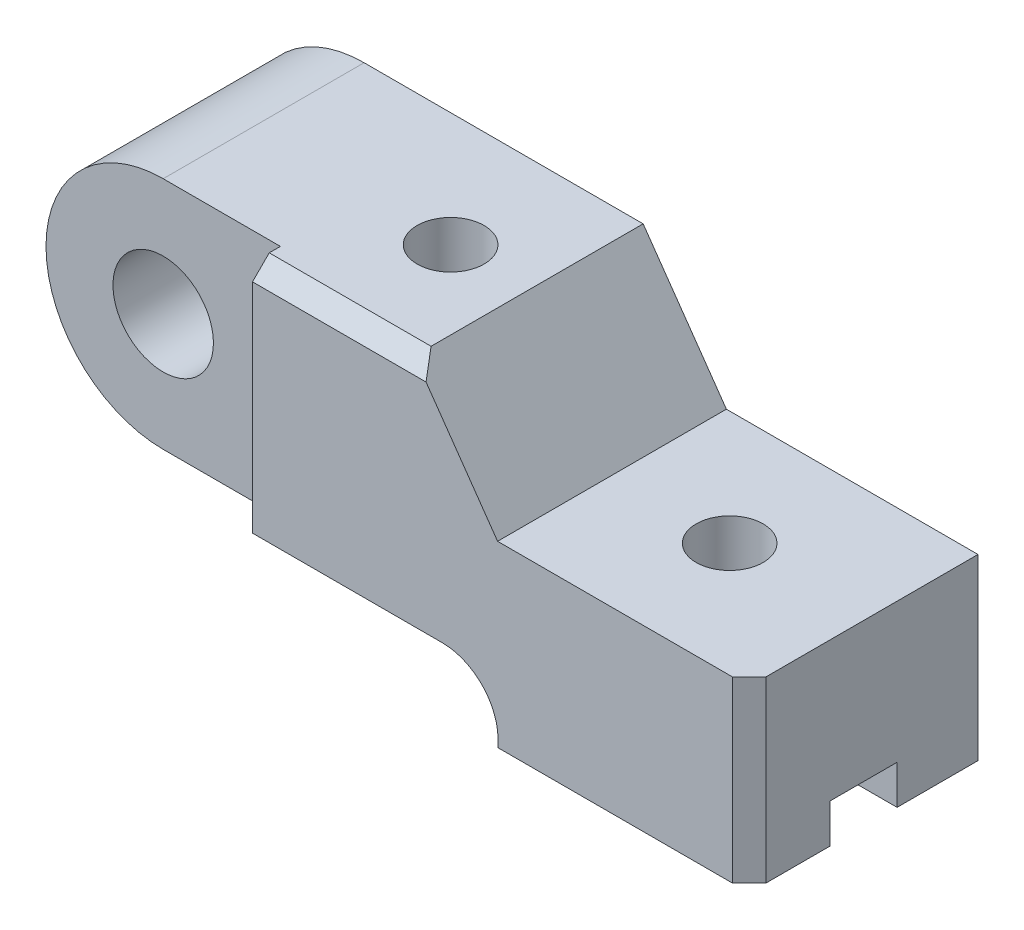
ISO-10303-21;
HEADER;
FILE_DESCRIPTION(('STEP AP214'),'2;1');
FILE_NAME('part.step','',(''),(''),'','','');
FILE_SCHEMA(('AUTOMOTIVE_DESIGN { 1 0 10303 214 1 1 1 1 }'));
ENDSEC;
DATA;
#1=APPLICATION_CONTEXT('core data for automotive mechanical design processes');
#2=APPLICATION_PROTOCOL_DEFINITION('international standard','automotive_design',2000,#1);
#3=PRODUCT_CONTEXT('',#1,'mechanical');
#4=PRODUCT('Part','Part','',(#3));
#5=PRODUCT_RELATED_PRODUCT_CATEGORY('part','',(#4));
#6=PRODUCT_DEFINITION_FORMATION('','',#4);
#7=PRODUCT_DEFINITION_CONTEXT('part definition',#1,'design');
#8=PRODUCT_DEFINITION('design','',#6,#7);
#9=PRODUCT_DEFINITION_SHAPE('','',#8);
#10=(LENGTH_UNIT() NAMED_UNIT(*) SI_UNIT(.MILLI.,.METRE.));
#11=(NAMED_UNIT(*) PLANE_ANGLE_UNIT() SI_UNIT($,.RADIAN.));
#12=(NAMED_UNIT(*) SI_UNIT($,.STERADIAN.) SOLID_ANGLE_UNIT());
#13=UNCERTAINTY_MEASURE_WITH_UNIT(LENGTH_MEASURE(1.E-05),#10,'distance_accuracy_value','');
#14=(GEOMETRIC_REPRESENTATION_CONTEXT(3) GLOBAL_UNCERTAINTY_ASSIGNED_CONTEXT((#13)) GLOBAL_UNIT_ASSIGNED_CONTEXT((#10,
#11,#12)) REPRESENTATION_CONTEXT('',''));
#15=CARTESIAN_POINT('',(0.,0.,0.));
#16=DIRECTION('',(0.,0.,1.));
#17=DIRECTION('',(1.,0.,0.));
#18=AXIS2_PLACEMENT_3D('',#15,#16,#17);
#19=CARTESIAN_POINT('',(-35.5,-25.305162605882,6.));
#20=DIRECTION('',(0.,1.,0.));
#21=DIRECTION('',(0.,0.,1.));
#22=AXIS2_PLACEMENT_3D('',#19,#20,#21);
#23=PLANE('',#22);
#24=DIRECTION('',(1.,0.,0.));
#25=VECTOR('',#24,1.);
#26=CARTESIAN_POINT('',(-35.5,-25.305162605882,6.));
#27=LINE('',#26,#25);
#28=CARTESIAN_POINT('',(86.,-25.3051626058819,6.));
#29=VERTEX_POINT('',#28);
#30=CARTESIAN_POINT('',(110.,-25.305162605882,6.));
#31=VERTEX_POINT('',#30);
#32=EDGE_CURVE('E184',#29,#31,#27,.T.);
#33=ORIENTED_EDGE('',*,*,#32,.F.);
#34=CARTESIAN_POINT('',(86.,-25.3051626058819,0.));
#35=DIRECTION('',(0.,1.,0.));
#36=DIRECTION('',(0.,0.,1.));
#37=AXIS2_PLACEMENT_3D('',#34,#35,#36);
#38=CIRCLE('',#37,6.);
#39=CARTESIAN_POINT('',(86.,-25.3051626058819,-6.00000000000001));
#40=VERTEX_POINT('',#39);
#41=EDGE_CURVE('E59',#29,#40,#38,.T.);
#42=ORIENTED_EDGE('',*,*,#41,.T.);
#43=DIRECTION('',(1.,0.,0.));
#44=VECTOR('',#43,1.);
#45=CARTESIAN_POINT('',(-35.5,-25.305162605882,-6.));
#46=LINE('',#45,#44);
#47=CARTESIAN_POINT('',(110.,-25.305162605882,-6.));
#48=VERTEX_POINT('',#47);
#49=EDGE_CURVE('E181',#40,#48,#46,.T.);
#50=ORIENTED_EDGE('',*,*,#49,.T.);
#51=DIRECTION('',(0.,0.,1.));
#52=VECTOR('',#51,1.);
#53=CARTESIAN_POINT('',(110.,-25.305162605882,6.));
#54=LINE('',#53,#52);
#55=EDGE_CURVE('E204',#48,#31,#54,.T.);
#56=ORIENTED_EDGE('',*,*,#55,.T.);
#57=EDGE_LOOP('',(#33,#42,#50,#56));
#58=FACE_BOUND('',#57,.T.);
#59=ADVANCED_FACE('F43',(#58),#23,.F.);
#60=CARTESIAN_POINT('',(65.,0.,20.5));
#61=DIRECTION('',(-1.,0.,0.));
#62=DIRECTION('',(0.,0.,1.));
#63=AXIS2_PLACEMENT_3D('',#60,#61,#62);
#64=PLANE('',#63);
#65=DIRECTION('',(0.,1.,0.));
#66=VECTOR('',#65,1.);
#67=CARTESIAN_POINT('',(65.,0.,6.));
#68=LINE('',#67,#66);
#69=CARTESIAN_POINT('',(65.,-32.305162605882,5.99999999999999));
#70=VERTEX_POINT('',#69);
#71=CARTESIAN_POINT('',(65.,-31.0000000000001,6.));
#72=VERTEX_POINT('',#71);
#73=EDGE_CURVE('E209',#70,#72,#68,.T.);
#74=ORIENTED_EDGE('',*,*,#73,.F.);
#75=DIRECTION('',(0.,0.,-1.));
#76=VECTOR('',#75,1.);
#77=CARTESIAN_POINT('',(65.,-32.305162605882,20.5));
#78=LINE('',#77,#76);
#79=CARTESIAN_POINT('',(65.,-32.305162605882,20.5));
#80=VERTEX_POINT('',#79);
#81=EDGE_CURVE('E297',#80,#70,#78,.T.);
#82=ORIENTED_EDGE('',*,*,#81,.F.);
#83=DIRECTION('',(0.,1.,0.));
#84=VECTOR('',#83,1.);
#85=CARTESIAN_POINT('',(65.,0.,20.5));
#86=LINE('',#85,#84);
#87=CARTESIAN_POINT('',(65.,-31.0000000000001,20.5));
#88=VERTEX_POINT('',#87);
#89=EDGE_CURVE('E250',#80,#88,#86,.T.);
#90=ORIENTED_EDGE('',*,*,#89,.T.);
#91=DIRECTION('',(0.,0.,-1.));
#92=VECTOR('',#91,1.);
#93=CARTESIAN_POINT('',(65.,-31.0000000000001,20.5));
#94=LINE('',#93,#92);
#95=EDGE_CURVE('E296',#88,#72,#94,.T.);
#96=ORIENTED_EDGE('',*,*,#95,.T.);
#97=EDGE_LOOP('',(#74,#82,#90,#96));
#98=FACE_BOUND('',#97,.T.);
#99=ADVANCED_FACE('F394',(#98),#64,.T.);
#100=CARTESIAN_POINT('',(0.,-32.305162605882,20.5));
#101=DIRECTION('',(0.,-1.,0.));
#102=DIRECTION('',(1.,0.,0.));
#103=AXIS2_PLACEMENT_3D('',#100,#101,#102);
#104=PLANE('',#103);
#105=DIRECTION('',(1.,0.,0.));
#106=VECTOR('',#105,1.);
#107=CARTESIAN_POINT('',(-35.5,-32.305162605882,5.99999999999999));
#108=LINE('',#107,#106);
#109=CARTESIAN_POINT('',(110.,-32.305162605882,5.99999999999999));
#110=VERTEX_POINT('',#109);
#111=EDGE_CURVE('E205',#70,#110,#108,.T.);
#112=ORIENTED_EDGE('',*,*,#111,.T.);
#113=DIRECTION('',(0.,0.,-1.));
#114=VECTOR('',#113,1.);
#115=CARTESIAN_POINT('',(110.,-32.305162605882,20.5));
#116=LINE('',#115,#114);
#117=CARTESIAN_POINT('',(110.,-32.305162605882,17.5));
#118=VERTEX_POINT('',#117);
#119=EDGE_CURVE('E295',#118,#110,#116,.T.);
#120=ORIENTED_EDGE('',*,*,#119,.F.);
#121=DIRECTION('',(0.707106781186548,0.,-0.707106781186548));
#122=VECTOR('',#121,1.);
#123=CARTESIAN_POINT('',(53.5,-32.305162605882,74.));
#124=LINE('',#123,#122);
#125=CARTESIAN_POINT('',(107.,-32.305162605882,20.5));
#126=VERTEX_POINT('',#125);
#127=EDGE_CURVE('E320',#118,#126,#124,.F.);
#128=ORIENTED_EDGE('',*,*,#127,.T.);
#129=DIRECTION('',(-1.,0.,0.));
#130=VECTOR('',#129,1.);
#131=CARTESIAN_POINT('',(0.,-32.305162605882,20.5));
#132=LINE('',#131,#130);
#133=EDGE_CURVE('E247',#126,#80,#132,.T.);
#134=ORIENTED_EDGE('',*,*,#133,.T.);
#135=ORIENTED_EDGE('',*,*,#81,.T.);
#136=EDGE_LOOP('',(#112,#120,#128,#134,#135));
#137=FACE_BOUND('',#136,.T.);
#138=ADVANCED_FACE('F339',(#137),#104,.T.);
#139=CARTESIAN_POINT('',(0.,-21.,20.5));
#140=DIRECTION('',(0.,-1.,0.));
#141=DIRECTION('',(0.,0.,-1.));
#142=AXIS2_PLACEMENT_3D('',#139,#140,#141);
#143=PLANE('',#142);
#144=CARTESIAN_POINT('',(36.,-21.,0.));
#145=DIRECTION('',(0.,-1.,0.));
#146=DIRECTION('',(0.,0.,-1.));
#147=AXIS2_PLACEMENT_3D('',#144,#145,#146);
#148=CIRCLE('',#147,6.);
#149=CARTESIAN_POINT('',(36.,-21.,-6.));
#150=VERTEX_POINT('',#149);
#151=EDGE_CURVE('E347',#150,#150,#148,.T.);
#152=ORIENTED_EDGE('',*,*,#151,.F.);
#153=EDGE_LOOP('',(#152));
#154=FACE_BOUND('',#153,.T.);
#155=DIRECTION('',(-1.,0.,0.));
#156=VECTOR('',#155,1.);
#157=CARTESIAN_POINT('',(0.,-21.,-20.5));
#158=LINE('',#157,#156);
#159=CARTESIAN_POINT('',(54.9999999999999,-21.,-20.5));
#160=VERTEX_POINT('',#159);
#161=CARTESIAN_POINT('',(0.,-21.,-20.5));
#162=VERTEX_POINT('',#161);
#163=EDGE_CURVE('E239',#160,#162,#158,.T.);
#164=ORIENTED_EDGE('',*,*,#163,.F.);
#165=DIRECTION('',(0.,0.,-1.));
#166=VECTOR('',#165,1.);
#167=CARTESIAN_POINT('',(54.9999999999999,-21.,20.5));
#168=LINE('',#167,#166);
#169=CARTESIAN_POINT('',(54.9999999999999,-21.,20.5));
#170=VERTEX_POINT('',#169);
#171=EDGE_CURVE('E301',#170,#160,#168,.T.);
#172=ORIENTED_EDGE('',*,*,#171,.F.);
#173=DIRECTION('',(-1.,0.,0.));
#174=VECTOR('',#173,1.);
#175=CARTESIAN_POINT('',(0.,-21.,20.5));
#176=LINE('',#175,#174);
#177=CARTESIAN_POINT('',(21.,-21.,20.5));
#178=VERTEX_POINT('',#177);
#179=EDGE_CURVE('E242',#170,#178,#176,.T.);
#180=ORIENTED_EDGE('',*,*,#179,.T.);
#181=DIRECTION('',(0.,0.,-1.));
#182=VECTOR('',#181,1.);
#183=CARTESIAN_POINT('',(21.,-21.,20.5));
#184=LINE('',#183,#182);
#185=CARTESIAN_POINT('',(21.,-21.,15.5));
#186=VERTEX_POINT('',#185);
#187=EDGE_CURVE('E259',#178,#186,#184,.T.);
#188=ORIENTED_EDGE('',*,*,#187,.T.);
#189=DIRECTION('',(-1.,0.,0.));
#190=VECTOR('',#189,1.);
#191=CARTESIAN_POINT('',(0.,-21.,15.5));
#192=LINE('',#191,#190);
#193=CARTESIAN_POINT('',(0.,-21.,15.5));
#194=VERTEX_POINT('',#193);
#195=EDGE_CURVE('E221',#186,#194,#192,.T.);
#196=ORIENTED_EDGE('',*,*,#195,.T.);
#197=DIRECTION('',(0.,0.,1.));
#198=VECTOR('',#197,1.);
#199=CARTESIAN_POINT('',(0.,-21.,-20.5));
#200=LINE('',#199,#198);
#201=EDGE_CURVE('E240',#162,#194,#200,.T.);
#202=ORIENTED_EDGE('',*,*,#201,.F.);
#203=EDGE_LOOP('',(#164,#172,#180,#188,#196,#202));
#204=FACE_BOUND('',#203,.T.);
#205=ADVANCED_FACE('F387',(#154,#204),#143,.T.);
#206=CARTESIAN_POINT('',(55.,-31.,20.5));
#207=DIRECTION('',(0.,0.,-1.));
#208=DIRECTION('',(-1.,0.,0.));
#209=AXIS2_PLACEMENT_3D('',#206,#207,#208);
#210=CYLINDRICAL_SURFACE('',#209,10.);
#211=DIRECTION('',(0.,0.,-1.));
#212=VECTOR('',#211,1.);
#213=CARTESIAN_POINT('',(63.2200259765134,-25.305162605882,20.5));
#214=LINE('',#213,#212);
#215=CARTESIAN_POINT('',(63.2200259765134,-25.305162605882,-6.));
#216=VERTEX_POINT('',#215);
#217=CARTESIAN_POINT('',(63.2200259765134,-25.305162605882,6.));
#218=VERTEX_POINT('',#217);
#219=EDGE_CURVE('E198',#216,#218,#214,.F.);
#220=ORIENTED_EDGE('',*,*,#219,.T.);
#221=CARTESIAN_POINT('',(55.,-31.,5.99999999999999));
#222=DIRECTION('',(0.,0.,1.));
#223=DIRECTION('',(0.,-1.,0.));
#224=AXIS2_PLACEMENT_3D('',#221,#222,#223);
#225=CIRCLE('',#224,10.);
#226=EDGE_CURVE('E215',#218,#72,#225,.F.);
#227=ORIENTED_EDGE('',*,*,#226,.T.);
#228=ORIENTED_EDGE('',*,*,#95,.F.);
#229=CARTESIAN_POINT('',(55.,-31.,20.5));
#230=DIRECTION('',(0.,0.,1.));
#231=DIRECTION('',(1.,0.,0.));
#232=AXIS2_PLACEMENT_3D('',#229,#230,#231);
#233=CIRCLE('',#232,10.);
#234=EDGE_CURVE('E244',#170,#88,#233,.F.);
#235=ORIENTED_EDGE('',*,*,#234,.F.);
#236=ORIENTED_EDGE('',*,*,#171,.T.);
#237=CARTESIAN_POINT('',(55.,-31.,-20.5));
#238=DIRECTION('',(0.,0.,1.));
#239=DIRECTION('',(1.,0.,0.));
#240=AXIS2_PLACEMENT_3D('',#237,#238,#239);
#241=CIRCLE('',#240,10.);
#242=CARTESIAN_POINT('',(65.,-31.0000000000001,-20.5));
#243=VERTEX_POINT('',#242);
#244=EDGE_CURVE('E261',#160,#243,#241,.F.);
#245=ORIENTED_EDGE('',*,*,#244,.T.);
#246=CARTESIAN_POINT('',(65.,-31.0000000000001,-6.00000000000001));
#247=VERTEX_POINT('',#246);
#248=EDGE_CURVE('E299',#247,#243,#94,.T.);
#249=ORIENTED_EDGE('',*,*,#248,.F.);
#250=CARTESIAN_POINT('',(55.,-31.,-6.00000000000001));
#251=DIRECTION('',(0.,0.,-1.));
#252=DIRECTION('',(0.,1.,0.));
#253=AXIS2_PLACEMENT_3D('',#250,#251,#252);
#254=CIRCLE('',#253,10.);
#255=EDGE_CURVE('E210',#247,#216,#254,.F.);
#256=ORIENTED_EDGE('',*,*,#255,.T.);
#257=EDGE_LOOP('',(#220,#227,#228,#235,#236,#245,#249,#256));
#258=FACE_BOUND('',#257,.T.);
#259=ADVANCED_FACE('F395',(#258),#210,.F.);
#260=DIRECTION('',(0.,-1.,0.));
#261=VECTOR('',#260,1.);
#262=CARTESIAN_POINT('',(65.,0.,-6.));
#263=LINE('',#262,#261);
#264=CARTESIAN_POINT('',(65.,-32.305162605882,-6.00000000000001));
#265=VERTEX_POINT('',#264);
#266=EDGE_CURVE('E202',#247,#265,#263,.T.);
#267=ORIENTED_EDGE('',*,*,#266,.F.);
#268=ORIENTED_EDGE('',*,*,#248,.T.);
#269=DIRECTION('',(0.,1.,0.));
#270=VECTOR('',#269,1.);
#271=CARTESIAN_POINT('',(65.,0.,-20.5));
#272=LINE('',#271,#270);
#273=CARTESIAN_POINT('',(65.,-32.305162605882,-20.5));
#274=VERTEX_POINT('',#273);
#275=EDGE_CURVE('E262',#274,#243,#272,.T.);
#276=ORIENTED_EDGE('',*,*,#275,.F.);
#277=EDGE_CURVE('E293',#265,#274,#78,.T.);
#278=ORIENTED_EDGE('',*,*,#277,.F.);
#279=EDGE_LOOP('',(#267,#268,#276,#278));
#280=FACE_BOUND('',#279,.T.);
#281=ADVANCED_FACE('F396',(#280),#64,.T.);
#282=DIRECTION('',(1.,0.,0.));
#283=VECTOR('',#282,1.);
#284=CARTESIAN_POINT('',(-35.5,-32.305162605882,-6.00000000000001));
#285=LINE('',#284,#283);
#286=CARTESIAN_POINT('',(110.,-32.305162605882,-6.));
#287=VERTEX_POINT('',#286);
#288=EDGE_CURVE('E68',#265,#287,#285,.T.);
#289=ORIENTED_EDGE('',*,*,#288,.F.);
#290=ORIENTED_EDGE('',*,*,#277,.T.);
#291=DIRECTION('',(-1.,0.,0.));
#292=VECTOR('',#291,1.);
#293=CARTESIAN_POINT('',(0.,-32.305162605882,-20.5));
#294=LINE('',#293,#292);
#295=CARTESIAN_POINT('',(110.,-32.305162605882,-20.5));
#296=VERTEX_POINT('',#295);
#297=EDGE_CURVE('E270',#296,#274,#294,.T.);
#298=ORIENTED_EDGE('',*,*,#297,.F.);
#299=EDGE_CURVE('E292',#287,#296,#116,.T.);
#300=ORIENTED_EDGE('',*,*,#299,.F.);
#301=EDGE_LOOP('',(#289,#290,#298,#300));
#302=FACE_BOUND('',#301,.T.);
#303=ADVANCED_FACE('F351',(#302),#104,.T.);
#304=CARTESIAN_POINT('',(110.,0.,20.5));
#305=DIRECTION('',(1.,0.,0.));
#306=DIRECTION('',(0.,0.,-1.));
#307=AXIS2_PLACEMENT_3D('',#304,#305,#306);
#308=PLANE('',#307);
#309=DIRECTION('',(0.,-1.,0.));
#310=VECTOR('',#309,1.);
#311=CARTESIAN_POINT('',(110.,-32.305162605882,5.99999999999999));
#312=LINE('',#311,#310);
#313=EDGE_CURVE('E344',#31,#110,#312,.T.);
#314=ORIENTED_EDGE('',*,*,#313,.F.);
#315=ORIENTED_EDGE('',*,*,#55,.F.);
#316=DIRECTION('',(0.,1.,0.));
#317=VECTOR('',#316,1.);
#318=CARTESIAN_POINT('',(110.,-32.305162605882,-6.00000000000001));
#319=LINE('',#318,#317);
#320=EDGE_CURVE('E193',#287,#48,#319,.T.);
#321=ORIENTED_EDGE('',*,*,#320,.F.);
#322=ORIENTED_EDGE('',*,*,#299,.T.);
#323=DIRECTION('',(0.,-1.,0.));
#324=VECTOR('',#323,1.);
#325=CARTESIAN_POINT('',(110.,0.,-20.5));
#326=LINE('',#325,#324);
#327=CARTESIAN_POINT('',(110.,-0.30516260588195,-20.5));
#328=VERTEX_POINT('',#327);
#329=EDGE_CURVE('E269',#328,#296,#326,.T.);
#330=ORIENTED_EDGE('',*,*,#329,.F.);
#331=DIRECTION('',(0.,0.,-1.));
#332=VECTOR('',#331,1.);
#333=CARTESIAN_POINT('',(110.,-0.30516260588195,20.5));
#334=LINE('',#333,#332);
#335=CARTESIAN_POINT('',(110.,-0.30516260588195,17.5));
#336=VERTEX_POINT('',#335);
#337=EDGE_CURVE('E289',#336,#328,#334,.T.);
#338=ORIENTED_EDGE('',*,*,#337,.F.);
#339=DIRECTION('',(0.,-1.,0.));
#340=VECTOR('',#339,1.);
#341=CARTESIAN_POINT('',(110.,0.,17.5));
#342=LINE('',#341,#340);
#343=EDGE_CURVE('E314',#336,#118,#342,.T.);
#344=ORIENTED_EDGE('',*,*,#343,.T.);
#345=ORIENTED_EDGE('',*,*,#119,.T.);
#346=EDGE_LOOP('',(#314,#315,#321,#322,#330,#338,#344,#345));
#347=FACE_BOUND('',#346,.T.);
#348=ADVANCED_FACE('F337',(#347),#308,.T.);
#349=CARTESIAN_POINT('',(0.,-0.30516260588196,20.5));
#350=DIRECTION('',(0.,1.,0.));
#351=DIRECTION('',(-1.,0.,0.));
#352=AXIS2_PLACEMENT_3D('',#349,#350,#351);
#353=PLANE('',#352);
#354=CARTESIAN_POINT('',(86.,-0.305162605881953,0.));
#355=DIRECTION('',(0.,1.,0.));
#356=DIRECTION('',(-1.,0.,0.));
#357=AXIS2_PLACEMENT_3D('',#354,#355,#356);
#358=CIRCLE('',#357,6.);
#359=CARTESIAN_POINT('',(80.,-0.305162605881954,0.));
#360=VERTEX_POINT('',#359);
#361=EDGE_CURVE('E187',#360,#360,#358,.T.);
#362=ORIENTED_EDGE('',*,*,#361,.F.);
#363=EDGE_LOOP('',(#362));
#364=FACE_BOUND('',#363,.T.);
#365=DIRECTION('',(1.,0.,0.));
#366=VECTOR('',#365,1.);
#367=CARTESIAN_POINT('',(0.,-0.30516260588196,20.5));
#368=LINE('',#367,#366);
#369=CARTESIAN_POINT('',(64.9180354594221,-0.305162605881953,20.5));
#370=VERTEX_POINT('',#369);
#371=CARTESIAN_POINT('',(107.,-0.305162605881951,20.5));
#372=VERTEX_POINT('',#371);
#373=EDGE_CURVE('E252',#370,#372,#368,.T.);
#374=ORIENTED_EDGE('',*,*,#373,.T.);
#375=DIRECTION('',(-0.707106781186548,0.,0.707106781186548));
#376=VECTOR('',#375,1.);
#377=CARTESIAN_POINT('',(53.5,-0.305162605881955,74.));
#378=LINE('',#377,#376);
#379=EDGE_CURVE('E11',#372,#336,#378,.F.);
#380=ORIENTED_EDGE('',*,*,#379,.T.);
#381=ORIENTED_EDGE('',*,*,#337,.T.);
#382=DIRECTION('',(1.,0.,0.));
#383=VECTOR('',#382,1.);
#384=CARTESIAN_POINT('',(0.,-0.30516260588196,-20.5));
#385=LINE('',#384,#383);
#386=CARTESIAN_POINT('',(64.9180354594221,-0.305162605881953,-20.5));
#387=VERTEX_POINT('',#386);
#388=EDGE_CURVE('E272',#387,#328,#385,.T.);
#389=ORIENTED_EDGE('',*,*,#388,.F.);
#390=DIRECTION('',(0.,0.,-1.));
#391=VECTOR('',#390,1.);
#392=CARTESIAN_POINT('',(64.9180354594221,-0.305162605881953,20.5));
#393=LINE('',#392,#391);
#394=EDGE_CURVE('E290',#370,#387,#393,.T.);
#395=ORIENTED_EDGE('',*,*,#394,.F.);
#396=EDGE_LOOP('',(#374,#380,#381,#389,#395));
#397=FACE_BOUND('',#396,.T.);
#398=ADVANCED_FACE('F328',(#364,#397),#353,.T.);
#399=CARTESIAN_POINT('',(43.4172761013938,30.4011040147281,20.5));
#400=DIRECTION('',(0.819152044288993,0.573576436351044,0.));
#401=DIRECTION('',(-0.573576436351044,0.819152044288993,0.));
#402=AXIS2_PLACEMENT_3D('',#399,#400,#401);
#403=PLANE('',#402);
#404=DIRECTION('',(0.,0.,-1.));
#405=VECTOR('',#404,1.);
#406=CARTESIAN_POINT('',(50.,21.,20.5));
#407=LINE('',#406,#405);
#408=CARTESIAN_POINT('',(50.,21.,17.5));
#409=VERTEX_POINT('',#408);
#410=CARTESIAN_POINT('',(50.,21.,-20.5));
#411=VERTEX_POINT('',#410);
#412=EDGE_CURVE('E281',#409,#411,#407,.T.);
#413=ORIENTED_EDGE('',*,*,#412,.F.);
#414=DIRECTION('',(-0.443712606279656,0.633687274224643,-0.633687274224643));
#415=VECTOR('',#414,1.);
#416=CARTESIAN_POINT('',(46.904156919725,25.4213221242812,13.0786778757188));
#417=LINE('',#416,#415);
#418=CARTESIAN_POINT('',(52.1006226146291,18.,20.5));
#419=VERTEX_POINT('',#418);
#420=EDGE_CURVE('E306',#409,#419,#417,.F.);
#421=ORIENTED_EDGE('',*,*,#420,.T.);
#422=DIRECTION('',(0.573576436351044,-0.819152044288993,0.));
#423=VECTOR('',#422,1.);
#424=CARTESIAN_POINT('',(43.4172761013938,30.4011040147281,20.5));
#425=LINE('',#424,#423);
#426=EDGE_CURVE('E254',#419,#370,#425,.T.);
#427=ORIENTED_EDGE('',*,*,#426,.T.);
#428=ORIENTED_EDGE('',*,*,#394,.T.);
#429=DIRECTION('',(0.573576436351044,-0.819152044288993,0.));
#430=VECTOR('',#429,1.);
#431=CARTESIAN_POINT('',(43.4172761013938,30.4011040147281,-20.5));
#432=LINE('',#431,#430);
#433=EDGE_CURVE('E277',#411,#387,#432,.T.);
#434=ORIENTED_EDGE('',*,*,#433,.F.);
#435=EDGE_LOOP('',(#413,#421,#427,#428,#434));
#436=FACE_BOUND('',#435,.T.);
#437=ADVANCED_FACE('F364',(#436),#403,.T.);
#438=CARTESIAN_POINT('',(0.,21.,20.5));
#439=DIRECTION('',(0.,1.,0.));
#440=DIRECTION('',(0.,0.,1.));
#441=AXIS2_PLACEMENT_3D('',#438,#439,#440);
#442=PLANE('',#441);
#443=CARTESIAN_POINT('',(36.,21.,0.));
#444=DIRECTION('',(0.,1.,0.));
#445=DIRECTION('',(0.,0.,1.));
#446=AXIS2_PLACEMENT_3D('',#443,#444,#445);
#447=CIRCLE('',#446,6.);
#448=CARTESIAN_POINT('',(36.,21.,6.));
#449=VERTEX_POINT('',#448);
#450=EDGE_CURVE('E176',#449,#449,#447,.T.);
#451=ORIENTED_EDGE('',*,*,#450,.F.);
#452=EDGE_LOOP('',(#451));
#453=FACE_BOUND('',#452,.T.);
#454=DIRECTION('',(0.,0.,-1.));
#455=VECTOR('',#454,1.);
#456=CARTESIAN_POINT('',(21.,21.,20.5));
#457=LINE('',#456,#455);
#458=CARTESIAN_POINT('',(21.,21.,17.5));
#459=VERTEX_POINT('',#458);
#460=CARTESIAN_POINT('',(21.,21.,15.5));
#461=VERTEX_POINT('',#460);
#462=EDGE_CURVE('E283',#459,#461,#457,.T.);
#463=ORIENTED_EDGE('',*,*,#462,.F.);
#464=DIRECTION('',(1.,0.,0.));
#465=VECTOR('',#464,1.);
#466=CARTESIAN_POINT('',(0.,21.,17.5));
#467=LINE('',#466,#465);
#468=EDGE_CURVE('E302',#459,#409,#467,.T.);
#469=ORIENTED_EDGE('',*,*,#468,.T.);
#470=ORIENTED_EDGE('',*,*,#412,.T.);
#471=DIRECTION('',(1.,0.,0.));
#472=VECTOR('',#471,1.);
#473=CARTESIAN_POINT('',(0.,21.,-20.5));
#474=LINE('',#473,#472);
#475=CARTESIAN_POINT('',(0.,21.,-20.5));
#476=VERTEX_POINT('',#475);
#477=EDGE_CURVE('E241',#476,#411,#474,.T.);
#478=ORIENTED_EDGE('',*,*,#477,.F.);
#479=DIRECTION('',(0.,0.,1.));
#480=VECTOR('',#479,1.);
#481=CARTESIAN_POINT('',(0.,21.,-20.5));
#482=LINE('',#481,#480);
#483=CARTESIAN_POINT('',(0.,21.,15.5));
#484=VERTEX_POINT('',#483);
#485=EDGE_CURVE('E237',#476,#484,#482,.T.);
#486=ORIENTED_EDGE('',*,*,#485,.T.);
#487=DIRECTION('',(1.,0.,0.));
#488=VECTOR('',#487,1.);
#489=CARTESIAN_POINT('',(0.,21.,15.5));
#490=LINE('',#489,#488);
#491=EDGE_CURVE('E217',#484,#461,#490,.T.);
#492=ORIENTED_EDGE('',*,*,#491,.T.);
#493=EDGE_LOOP('',(#463,#469,#470,#478,#486,#492));
#494=FACE_BOUND('',#493,.T.);
#495=ADVANCED_FACE('F380',(#453,#494),#442,.T.);
#496=CARTESIAN_POINT('',(21.,0.,20.5));
#497=DIRECTION('',(1.,0.,0.));
#498=DIRECTION('',(0.,0.,-1.));
#499=AXIS2_PLACEMENT_3D('',#496,#497,#498);
#500=PLANE('',#499);
#501=DIRECTION('',(0.,-1.,0.));
#502=VECTOR('',#501,1.);
#503=CARTESIAN_POINT('',(21.,0.,20.5));
#504=LINE('',#503,#502);
#505=CARTESIAN_POINT('',(21.,18.,20.5));
#506=VERTEX_POINT('',#505);
#507=EDGE_CURVE('E260',#506,#178,#504,.T.);
#508=ORIENTED_EDGE('',*,*,#507,.F.);
#509=DIRECTION('',(0.,-0.707106781186548,0.707106781186548));
#510=VECTOR('',#509,1.);
#511=CARTESIAN_POINT('',(21.,21.,17.5));
#512=LINE('',#511,#510);
#513=EDGE_CURVE('E315',#506,#459,#512,.F.);
#514=ORIENTED_EDGE('',*,*,#513,.T.);
#515=ORIENTED_EDGE('',*,*,#462,.T.);
#516=DIRECTION('',(0.,-1.,0.));
#517=VECTOR('',#516,1.);
#518=CARTESIAN_POINT('',(21.,0.,15.5));
#519=LINE('',#518,#517);
#520=EDGE_CURVE('E230',#461,#186,#519,.T.);
#521=ORIENTED_EDGE('',*,*,#520,.T.);
#522=ORIENTED_EDGE('',*,*,#187,.F.);
#523=EDGE_LOOP('',(#508,#514,#515,#521,#522));
#524=FACE_BOUND('',#523,.T.);
#525=ADVANCED_FACE('F372',(#524),#500,.F.);
#526=CARTESIAN_POINT('',(0.,0.,20.5));
#527=DIRECTION('',(0.,0.,1.));
#528=DIRECTION('',(1.,0.,0.));
#529=AXIS2_PLACEMENT_3D('',#526,#527,#528);
#530=PLANE('',#529);
#531=ORIENTED_EDGE('',*,*,#133,.F.);
#532=DIRECTION('',(0.,1.,0.));
#533=VECTOR('',#532,1.);
#534=CARTESIAN_POINT('',(107.,0.,20.5));
#535=LINE('',#534,#533);
#536=EDGE_CURVE('E55',#126,#372,#535,.T.);
#537=ORIENTED_EDGE('',*,*,#536,.T.);
#538=ORIENTED_EDGE('',*,*,#373,.F.);
#539=ORIENTED_EDGE('',*,*,#426,.F.);
#540=DIRECTION('',(-1.,0.,0.));
#541=VECTOR('',#540,1.);
#542=CARTESIAN_POINT('',(0.,18.,20.5));
#543=LINE('',#542,#541);
#544=EDGE_CURVE('E309',#419,#506,#543,.T.);
#545=ORIENTED_EDGE('',*,*,#544,.T.);
#546=ORIENTED_EDGE('',*,*,#507,.T.);
#547=ORIENTED_EDGE('',*,*,#179,.F.);
#548=ORIENTED_EDGE('',*,*,#234,.T.);
#549=ORIENTED_EDGE('',*,*,#89,.F.);
#550=EDGE_LOOP('',(#531,#537,#538,#539,#545,#546,#547,#548,#549));
#551=FACE_BOUND('',#550,.T.);
#552=ADVANCED_FACE('F325',(#551),#530,.T.);
#553=CARTESIAN_POINT('',(0.,0.,-20.5));
#554=DIRECTION('',(0.,0.,1.));
#555=DIRECTION('',(1.,0.,0.));
#556=AXIS2_PLACEMENT_3D('',#553,#554,#555);
#557=PLANE('',#556);
#558=ORIENTED_EDGE('',*,*,#163,.T.);
#559=CARTESIAN_POINT('',(0.,0.,-20.5));
#560=DIRECTION('',(0.,0.,1.));
#561=DIRECTION('',(1.,0.,0.));
#562=AXIS2_PLACEMENT_3D('',#559,#560,#561);
#563=CIRCLE('',#562,21.);
#564=EDGE_CURVE('E231',#476,#162,#563,.T.);
#565=ORIENTED_EDGE('',*,*,#564,.F.);
#566=ORIENTED_EDGE('',*,*,#477,.T.);
#567=ORIENTED_EDGE('',*,*,#433,.T.);
#568=ORIENTED_EDGE('',*,*,#388,.T.);
#569=ORIENTED_EDGE('',*,*,#329,.T.);
#570=ORIENTED_EDGE('',*,*,#297,.T.);
#571=ORIENTED_EDGE('',*,*,#275,.T.);
#572=ORIENTED_EDGE('',*,*,#244,.F.);
#573=EDGE_LOOP('',(#558,#565,#566,#567,#568,#569,#570,#571,#572));
#574=FACE_BOUND('',#573,.T.);
#575=CARTESIAN_POINT('',(0.,0.,-20.5));
#576=DIRECTION('',(0.,0.,1.));
#577=DIRECTION('',(1.,0.,0.));
#578=AXIS2_PLACEMENT_3D('',#575,#576,#577);
#579=CIRCLE('',#578,9.);
#580=CARTESIAN_POINT('',(9.,0.,-20.5));
#581=VERTEX_POINT('',#580);
#582=EDGE_CURVE('E226',#581,#581,#579,.T.);
#583=ORIENTED_EDGE('',*,*,#582,.T.);
#584=EDGE_LOOP('',(#583));
#585=FACE_BOUND('',#584,.T.);
#586=ADVANCED_FACE('F359',(#574,#585),#557,.F.);
#587=CARTESIAN_POINT('',(0.,0.,-20.5));
#588=DIRECTION('',(0.,0.,1.));
#589=DIRECTION('',(1.,0.,0.));
#590=AXIS2_PLACEMENT_3D('',#587,#588,#589);
#591=CYLINDRICAL_SURFACE('',#590,9.);
#592=ORIENTED_EDGE('',*,*,#582,.F.);
#593=EDGE_LOOP('',(#592));
#594=FACE_BOUND('',#593,.T.);
#595=CARTESIAN_POINT('',(0.,0.,15.5));
#596=DIRECTION('',(0.,0.,1.));
#597=DIRECTION('',(1.,0.,0.));
#598=AXIS2_PLACEMENT_3D('',#595,#596,#597);
#599=CIRCLE('',#598,9.);
#600=CARTESIAN_POINT('',(9.,0.,15.5));
#601=VERTEX_POINT('',#600);
#602=EDGE_CURVE('E214',#601,#601,#599,.T.);
#603=ORIENTED_EDGE('',*,*,#602,.T.);
#604=EDGE_LOOP('',(#603));
#605=FACE_BOUND('',#604,.T.);
#606=ADVANCED_FACE('F401',(#594,#605),#591,.F.);
#607=CARTESIAN_POINT('',(0.,0.,-20.5));
#608=DIRECTION('',(0.,0.,1.));
#609=DIRECTION('',(1.,0.,0.));
#610=AXIS2_PLACEMENT_3D('',#607,#608,#609);
#611=CYLINDRICAL_SURFACE('',#610,21.);
#612=ORIENTED_EDGE('',*,*,#201,.T.);
#613=CARTESIAN_POINT('',(0.,0.,15.5));
#614=DIRECTION('',(0.,0.,1.));
#615=DIRECTION('',(1.,0.,0.));
#616=AXIS2_PLACEMENT_3D('',#613,#614,#615);
#617=CIRCLE('',#616,21.);
#618=EDGE_CURVE('E222',#484,#194,#617,.T.);
#619=ORIENTED_EDGE('',*,*,#618,.F.);
#620=ORIENTED_EDGE('',*,*,#485,.F.);
#621=ORIENTED_EDGE('',*,*,#564,.T.);
#622=EDGE_LOOP('',(#612,#619,#620,#621));
#623=FACE_BOUND('',#622,.T.);
#624=ADVANCED_FACE('F402',(#623),#611,.T.);
#625=CARTESIAN_POINT('',(0.,0.,15.5));
#626=DIRECTION('',(0.,0.,1.));
#627=DIRECTION('',(1.,0.,0.));
#628=AXIS2_PLACEMENT_3D('',#625,#626,#627);
#629=PLANE('',#628);
#630=ORIENTED_EDGE('',*,*,#602,.F.);
#631=EDGE_LOOP('',(#630));
#632=FACE_BOUND('',#631,.T.);
#633=ORIENTED_EDGE('',*,*,#491,.F.);
#634=ORIENTED_EDGE('',*,*,#618,.T.);
#635=ORIENTED_EDGE('',*,*,#195,.F.);
#636=ORIENTED_EDGE('',*,*,#520,.F.);
#637=EDGE_LOOP('',(#633,#634,#635,#636));
#638=FACE_BOUND('',#637,.T.);
#639=ADVANCED_FACE('F382',(#632,#638),#629,.T.);
#640=CARTESIAN_POINT('',(0.,21.,17.5));
#641=DIRECTION('',(0.,-0.707106781186547,-0.707106781186547));
#642=DIRECTION('',(1.,0.,0.));
#643=AXIS2_PLACEMENT_3D('',#640,#641,#642);
#644=PLANE('',#643);
#645=ORIENTED_EDGE('',*,*,#513,.F.);
#646=ORIENTED_EDGE('',*,*,#544,.F.);
#647=ORIENTED_EDGE('',*,*,#420,.F.);
#648=ORIENTED_EDGE('',*,*,#468,.F.);
#649=EDGE_LOOP('',(#645,#646,#647,#648));
#650=FACE_BOUND('',#649,.T.);
#651=ADVANCED_FACE('F367',(#650),#644,.F.);
#652=CARTESIAN_POINT('',(110.,0.,17.5));
#653=DIRECTION('',(-0.707106781186547,0.,-0.707106781186547));
#654=DIRECTION('',(0.,-1.,0.));
#655=AXIS2_PLACEMENT_3D('',#652,#653,#654);
#656=PLANE('',#655);
#657=ORIENTED_EDGE('',*,*,#379,.F.);
#658=ORIENTED_EDGE('',*,*,#536,.F.);
#659=ORIENTED_EDGE('',*,*,#127,.F.);
#660=ORIENTED_EDGE('',*,*,#343,.F.);
#661=EDGE_LOOP('',(#657,#658,#659,#660));
#662=FACE_BOUND('',#661,.T.);
#663=ADVANCED_FACE('F46',(#662),#656,.F.);
#664=CARTESIAN_POINT('',(-35.5,-32.305162605882,5.99999999999999));
#665=DIRECTION('',(0.,0.,1.));
#666=DIRECTION('',(0.,-1.,0.));
#667=AXIS2_PLACEMENT_3D('',#664,#665,#666);
#668=PLANE('',#667);
#669=ORIENTED_EDGE('',*,*,#313,.T.);
#670=ORIENTED_EDGE('',*,*,#111,.F.);
#671=ORIENTED_EDGE('',*,*,#73,.T.);
#672=ORIENTED_EDGE('',*,*,#226,.F.);
#673=EDGE_CURVE('E197',#218,#29,#27,.T.);
#674=ORIENTED_EDGE('',*,*,#673,.T.);
#675=ORIENTED_EDGE('',*,*,#32,.T.);
#676=EDGE_LOOP('',(#669,#670,#671,#672,#674,#675));
#677=FACE_BOUND('',#676,.T.);
#678=ADVANCED_FACE('F342',(#677),#668,.F.);
#679=EDGE_CURVE('E189',#216,#40,#46,.T.);
#680=ORIENTED_EDGE('',*,*,#679,.T.);
#681=EDGE_CURVE('E175',#40,#29,#38,.T.);
#682=ORIENTED_EDGE('',*,*,#681,.T.);
#683=ORIENTED_EDGE('',*,*,#673,.F.);
#684=ORIENTED_EDGE('',*,*,#219,.F.);
#685=EDGE_LOOP('',(#680,#682,#683,#684));
#686=FACE_BOUND('',#685,.T.);
#687=ADVANCED_FACE('F194',(#686),#23,.F.);
#688=CARTESIAN_POINT('',(-35.5,-32.305162605882,-6.00000000000001));
#689=DIRECTION('',(0.,0.,-1.));
#690=DIRECTION('',(0.,1.,0.));
#691=AXIS2_PLACEMENT_3D('',#688,#689,#690);
#692=PLANE('',#691);
#693=ORIENTED_EDGE('',*,*,#288,.T.);
#694=ORIENTED_EDGE('',*,*,#320,.T.);
#695=ORIENTED_EDGE('',*,*,#49,.F.);
#696=ORIENTED_EDGE('',*,*,#679,.F.);
#697=ORIENTED_EDGE('',*,*,#255,.F.);
#698=ORIENTED_EDGE('',*,*,#266,.T.);
#699=EDGE_LOOP('',(#693,#694,#695,#696,#697,#698));
#700=FACE_BOUND('',#699,.T.);
#701=ADVANCED_FACE('F188',(#700),#692,.F.);
#702=CARTESIAN_POINT('',(86.,-134.5,0.));
#703=DIRECTION('',(0.,1.,0.));
#704=DIRECTION('',(0.,0.,1.));
#705=AXIS2_PLACEMENT_3D('',#702,#703,#704);
#706=CYLINDRICAL_SURFACE('',#705,6.);
#707=ORIENTED_EDGE('',*,*,#361,.T.);
#708=EDGE_LOOP('',(#707));
#709=FACE_BOUND('',#708,.T.);
#710=ORIENTED_EDGE('',*,*,#681,.F.);
#711=ORIENTED_EDGE('',*,*,#41,.F.);
#712=EDGE_LOOP('',(#710,#711));
#713=FACE_BOUND('',#712,.T.);
#714=ADVANCED_FACE('F173',(#709,#713),#706,.F.);
#715=CARTESIAN_POINT('',(36.,-134.5,0.));
#716=DIRECTION('',(0.,1.,0.));
#717=DIRECTION('',(0.,0.,1.));
#718=AXIS2_PLACEMENT_3D('',#715,#716,#717);
#719=CYLINDRICAL_SURFACE('',#718,6.);
#720=ORIENTED_EDGE('',*,*,#151,.T.);
#721=EDGE_LOOP('',(#720));
#722=FACE_BOUND('',#721,.T.);
#723=ORIENTED_EDGE('',*,*,#450,.T.);
#724=EDGE_LOOP('',(#723));
#725=FACE_BOUND('',#724,.T.);
#726=ADVANCED_FACE('F559',(#722,#725),#719,.F.);
#727=CLOSED_SHELL('',(#59,#99,#138,#205,#259,#281,#303,#348,#398,#437,#495,#525,#552,#586,#606,
#624,#639,#651,#663,#678,#687,#701,#714,#726));
#728=MANIFOLD_SOLID_BREP('B2',#727);
#729=ADVANCED_BREP_SHAPE_REPRESENTATION('',(#18,#728),#14);
#730=SHAPE_DEFINITION_REPRESENTATION(#9,#729);
ENDSEC;
END-ISO-10303-21;
